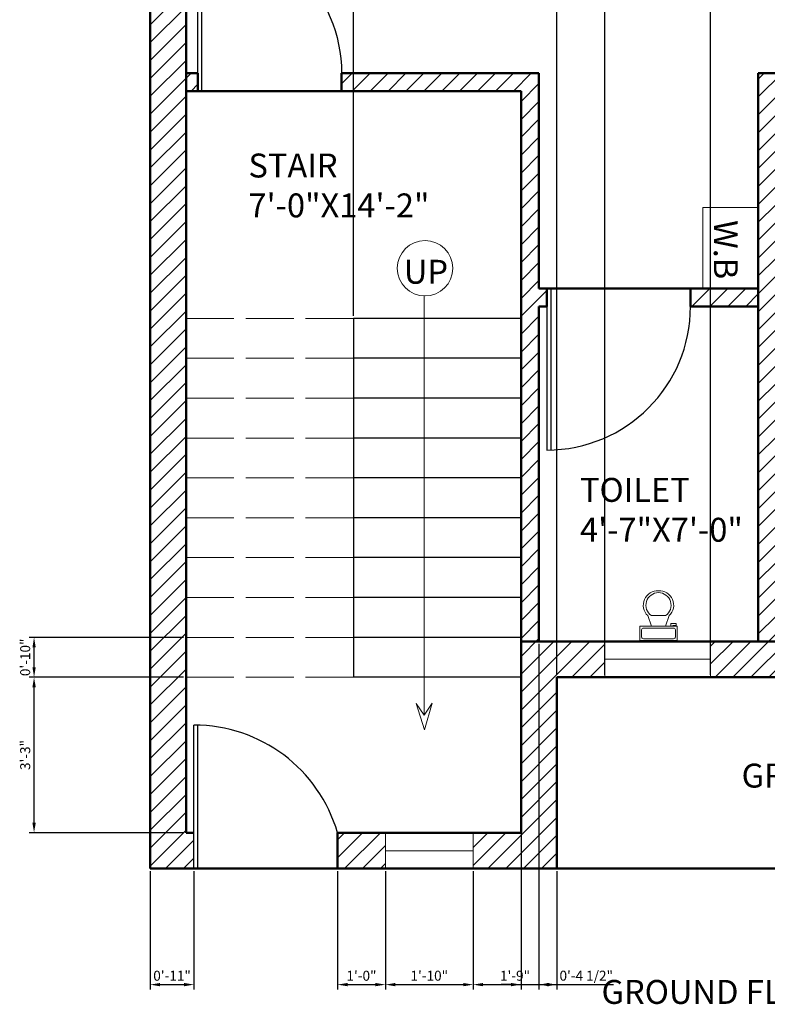
# Model space of a CAD drawing. Units: inches. Extents: x 3887 to 4286, y 884 to 1458.
# Tile 1 of 4: x 3889 to 4077, y 884 to 1131. Entities that reach past the tile are written whole.
import ezdxf

# ---------------------------------------------------------------- set-up
doc = ezdxf.new("R2010")
doc.units = ezdxf.units.IN
doc.linetypes.add('ACAD_ISO02W100', pattern=[15, 12, -3])
for name, color, linetype, lineweight in [('A-ANNO-DIMS', 2, 'Continuous', 18), ('A-ANNO-SYMB', 7, 'Continuous', 18), ('A-ANNO-TEXT', 7, 'Continuous', 25), ('A-AREA-IDEN', 7, 'Continuous', 25), ('A-DOOR', 3, 'Continuous', 25), ('A-FLOR-FIXT', 8, 'Continuous', 18), ('A-FLOR-STRS', 7, 'Continuous', 25), ('A-FLOR-STRS-OVHD', 8, 'ACAD_ISO02W100', 18), ('A-GLAZ', 4, 'Continuous', 18), ('A-WALL', 7, 'Continuous', 50), ('A-WALL-PATT', 252, 'Continuous', 13)]:
    doc.layers.add(name, color=color, linetype=linetype, lineweight=lineweight)
doc.styles.get("Standard").update_dxf_attribs({"font": 'arial.ttf'})
doc.dimstyles.new('ISO-25', dxfattribs={"dimtxt": 2.5, "dimasz": 2.5, "dimexe": 1.25, "dimexo": 0.625, "dimtad": 1, "dimdec": 0, "dimlunit": 3, "dimtxsty": 'Standard', "dimcen": 2.5, "dimadec": 0, "dimazin": 0, "dimtfac": 1, "dimtdec": 0, "dimtmove": 0, "dimatfit": 3, "dimfxl": 1, "dimarcsym": 0})

# ---------------------------------------------------------------- blocks, each defined once
blk = doc.blocks.new('*U5')
for p, q in [((9.5, -6), (9.5, -2)), ((-10, -8.5), (-8, -8.5)), ((-10, -9.5), (-10, -8.5)), ((-7, -9.5), (-10, -9.5)), ((-8, -8.5), (-8, -8)), ((-7, -8), (-7, -9.5)), ((-4, -8), (-6, -14)), ((4, -8), (6, -14)), ((4, -14), (-4, -14))]:
    blk.add_line(p, q)
blk.add_lwpolyline([(10.5, -8), (10.5, 0), (-10.5, 0), (-10.5, -8)], close=True)
for points in [[(-9.5, -2), (-9.5, -6)], [(8.5, -1), (-8.5, -1)], [(-8.5, -7), (8.5, -7)]]:
    blk.add_lwpolyline(points)
for centre, radius, start, end in [((-8.625, -1.875), 0.8839, 81.8699, 188.1301), ((8.625, -1.875), 0.8839, 351.8699, 98.1301), ((-8.625, -6.125), 0.8839, 171.869898, 278.1301), ((8.625, -6.125), 0.8839, 261.8699, 8.1301), ((-0.4772, -19.9188), 8.0953, 133.01722, 273.38), ((0.0374, -19.8731), 7.127, 124.50543, 269.7), ((-0.0373, -19.8731), 7.127, 270.3, 55.4946), ((0.4773, -19.9188), 8.0953, 266.62, 46.9828)]:
    blk.add_arc(centre, radius, start, end)
blk = doc.blocks.new('DOOR-SWING-36IN')
for p, q in [((35, 0), (35, 40.5)), ((36, 4.5), (36, 40.5))]:
    blk.add_line(p, q)
blk.add_arc((36, 4.5), 36, 90, 180)
blk = doc.blocks.new('*D39')
at = {"layer": 'A-ANNO-DIMS', "color": 0, "lineweight": -2, "transparency": 16777216}
for p, q in [((4015.18, 974.02), (4015.18, 887.29)), ((4019.68, 974.02), (4019.68, 887.29)), ((4012.68, 888.54), (4010.18, 888.54)), ((4015.18, 888.54), (4019.68, 888.54)), ((4022.18, 888.54), (4038.41, 888.54))]:
    blk.add_line(p, q, dxfattribs=at)
at = {"layer": 'A-ANNO-DIMS', "color": 0, "transparency": 16777216}
for points in [[(4012.68, 888.96), (4012.68, 888.13), (4015.18, 888.54)], [(4022.18, 888.96), (4022.18, 888.13), (4019.68, 888.54)]]:
    blk.add_solid(points, dxfattribs=at)
at = {"layer": 'Defpoints', "color": 0, "transparency": 16777216}
for p in [(4015.18, 974.64), (4019.68, 974.64), (4019.68, 888.54)]:
    blk.add_point(p, dxfattribs=at)
at = {"layer": 'A-ANNO-DIMS', "color": 0, "transparency": 16777216, "insert": (4031.54, 890.46), "char_height": 2.5, "attachment_point": 5}
blk.add_mtext('0\'-4 1/2"', dxfattribs=at)
blk = doc.blocks.new('*D40')
at = {"layer": 'A-ANNO-DIMS', "color": 0, "lineweight": -2, "transparency": 16777216}
for p, q in [((3922.18, 917.02), (3922.18, 887.29)), ((3933.18, 917.02), (3933.18, 887.29)), ((3924.68, 888.54), (3930.68, 888.54))]:
    blk.add_line(p, q, dxfattribs=at)
at = {"layer": 'A-ANNO-DIMS', "color": 0, "transparency": 16777216}
for points in [[(3924.68, 888.96), (3924.68, 888.13), (3922.18, 888.54)], [(3930.68, 888.96), (3930.68, 888.13), (3933.18, 888.54)]]:
    blk.add_solid(points, dxfattribs=at)
at = {"layer": 'Defpoints', "color": 0, "transparency": 16777216}
for p in [(3922.18, 917.64), (3933.18, 917.64), (3933.18, 888.54)]:
    blk.add_point(p, dxfattribs=at)
at = {"layer": 'A-ANNO-DIMS', "color": 0, "transparency": 16777216, "insert": (3927.68, 890.45), "char_height": 2.5, "attachment_point": 5}
blk.add_mtext('0\'-11"', dxfattribs=at)
blk = doc.blocks.new('*D41')
at = {"layer": 'A-ANNO-DIMS', "color": 0, "lineweight": -2, "transparency": 16777216}
for p, q in [((3969.18, 917.02), (3969.18, 887.29)), ((3981.18, 917.02), (3981.18, 887.29)), ((3971.68, 888.54), (3978.68, 888.54))]:
    blk.add_line(p, q, dxfattribs=at)
at = {"layer": 'A-ANNO-DIMS', "color": 0, "transparency": 16777216}
for points in [[(3971.68, 888.96), (3971.68, 888.13), (3969.18, 888.54)], [(3978.68, 888.96), (3978.68, 888.13), (3981.18, 888.54)]]:
    blk.add_solid(points, dxfattribs=at)
at = {"layer": 'Defpoints', "color": 0, "transparency": 16777216}
for p in [(3969.18, 917.64), (3981.18, 917.64), (3981.18, 888.54)]:
    blk.add_point(p, dxfattribs=at)
at = {"layer": 'A-ANNO-DIMS', "color": 0, "transparency": 16777216, "insert": (3975.18, 890.45), "char_height": 2.5, "attachment_point": 5}
blk.add_mtext('1\'-0"', dxfattribs=at)
blk = doc.blocks.new('*D43')
at = {"layer": 'A-ANNO-DIMS', "color": 0, "lineweight": -2, "transparency": 16777216}
for p, q in [((3981.18, 917.02), (3981.18, 887.29)), ((4003.18, 917.02), (4003.18, 887.29)), ((3983.68, 888.54), (4000.68, 888.54))]:
    blk.add_line(p, q, dxfattribs=at)
at = {"layer": 'A-ANNO-DIMS', "color": 0, "transparency": 16777216}
for points in [[(3983.68, 888.96), (3983.68, 888.13), (3981.18, 888.54)], [(4000.68, 888.96), (4000.68, 888.13), (4003.18, 888.54)]]:
    blk.add_solid(points, dxfattribs=at)
at = {"layer": 'Defpoints', "color": 0, "transparency": 16777216}
for p in [(3981.18, 917.64), (4003.18, 917.64), (4003.18, 888.54)]:
    blk.add_point(p, dxfattribs=at)
at = {"layer": 'A-ANNO-DIMS', "color": 0, "transparency": 16777216, "insert": (3992.18, 890.45), "char_height": 2.5, "attachment_point": 5}
blk.add_mtext('1\'-10"', dxfattribs=at)
blk = doc.blocks.new('*D44')
at = {"layer": 'A-ANNO-DIMS', "color": 0, "lineweight": -2, "transparency": 16777216}
for p, q in [((4003.18, 917.02), (4003.18, 887.29)), ((4024.18, 917.02), (4024.18, 887.29)), ((4005.68, 888.54), (4021.68, 888.54))]:
    blk.add_line(p, q, dxfattribs=at)
at = {"layer": 'A-ANNO-DIMS', "color": 0, "transparency": 16777216}
for points in [[(4005.68, 888.96), (4005.68, 888.13), (4003.18, 888.54)], [(4021.68, 888.96), (4021.68, 888.13), (4024.18, 888.54)]]:
    blk.add_solid(points, dxfattribs=at)
at = {"layer": 'Defpoints', "color": 0, "transparency": 16777216}
for p in [(4003.18, 917.64), (4024.18, 917.64), (4024.18, 888.54)]:
    blk.add_point(p, dxfattribs=at)
at = {"layer": 'A-ANNO-DIMS', "color": 0, "transparency": 16777216, "insert": (4013.68, 890.45), "char_height": 2.5, "attachment_point": 5}
blk.add_mtext('1\'-9"', dxfattribs=at)
blk = doc.blocks.new('*D45')
at = {"layer": 'A-ANNO-DIMS', "color": 0, "lineweight": -2, "transparency": 16777216}
for p, q in [((4024.18, 966.27), (4024.18, 1424.99)), ((4026.68, 1423.74), (4033.68, 1423.74)), ((4036.18, 966.27), (4036.18, 1424.99))]:
    blk.add_line(p, q, dxfattribs=at)
at = {"layer": 'A-ANNO-DIMS', "color": 0, "transparency": 16777216}
for points in [[(4026.68, 1424.16), (4026.68, 1423.33), (4024.18, 1423.74)], [(4033.68, 1424.16), (4033.68, 1423.33), (4036.18, 1423.74)]]:
    blk.add_solid(points, dxfattribs=at)
at = {"layer": 'Defpoints', "color": 0, "transparency": 16777216}
for p in [(4036.18, 1423.74), (4024.18, 965.64), (4036.18, 965.64)]:
    blk.add_point(p, dxfattribs=at)
at = {"layer": 'A-ANNO-DIMS', "color": 0, "transparency": 16777216, "insert": (4030.18, 1425.65), "char_height": 2.5, "attachment_point": 5}
blk.add_mtext('1\'-0"', dxfattribs=at)
blk = doc.blocks.new('*D46')
at = {"layer": 'A-ANNO-DIMS', "color": 0, "lineweight": -2, "transparency": 16777216}
for p, q in [((4036.18, 966.27), (4036.18, 1424.99)), ((4038.68, 1423.74), (4060.18, 1423.74)), ((4062.68, 966.27), (4062.68, 1424.99))]:
    blk.add_line(p, q, dxfattribs=at)
at = {"layer": 'A-ANNO-DIMS', "color": 0, "transparency": 16777216}
for points in [[(4038.68, 1424.16), (4038.68, 1423.33), (4036.18, 1423.74)], [(4060.18, 1424.16), (4060.18, 1423.33), (4062.68, 1423.74)]]:
    blk.add_solid(points, dxfattribs=at)
at = {"layer": 'Defpoints', "color": 0, "transparency": 16777216}
for p in [(4062.68, 1423.74), (4036.18, 965.64), (4062.68, 965.64)]:
    blk.add_point(p, dxfattribs=at)
at = {"layer": 'A-ANNO-DIMS', "color": 0, "transparency": 16777216, "insert": (4049.43, 1425.66), "char_height": 2.5, "attachment_point": 5}
blk.add_mtext('2\'-2 1/2"', dxfattribs=at)
blk = doc.blocks.new('*D47')
at = {"layer": 'A-ANNO-DIMS', "color": 0, "lineweight": -2, "transparency": 16777216}
for p, q in [((3930.56, 975.64), (3891.83, 975.64)), ((3893.08, 968.14), (3893.08, 973.14)), ((3930.56, 965.64), (3891.83, 965.64))]:
    blk.add_line(p, q, dxfattribs=at)
at = {"layer": 'A-ANNO-DIMS', "color": 0, "transparency": 16777216}
for points in [[(3892.67, 973.14), (3893.5, 973.14), (3893.08, 975.64)], [(3892.67, 968.14), (3893.5, 968.14), (3893.08, 965.64)]]:
    blk.add_solid(points, dxfattribs=at)
at = {"layer": 'Defpoints', "color": 0, "transparency": 16777216}
for p in [(3893.08, 975.64), (3931.18, 975.64), (3931.18, 965.64)]:
    blk.add_point(p, dxfattribs=at)
at = {"layer": 'A-ANNO-DIMS', "color": 0, "transparency": 16777216, "insert": (3891.18, 970.64), "char_height": 2.5, "attachment_point": 5, "rotation": 90}
blk.add_mtext('0\'-10"', dxfattribs=at)
blk = doc.blocks.new('*D52')
at = {"layer": 'A-ANNO-DIMS', "color": 0, "lineweight": -2, "transparency": 16777216}
for p, q in [((3931.18, 1056.27), (3931.18, 1424.99)), ((3933.68, 1423.74), (3970.68, 1423.74)), ((3973.18, 1056.27), (3973.18, 1424.99))]:
    blk.add_line(p, q, dxfattribs=at)
at = {"layer": 'A-ANNO-DIMS', "color": 0, "transparency": 16777216}
for points in [[(3933.68, 1424.16), (3933.68, 1423.33), (3931.18, 1423.74)], [(3970.68, 1424.16), (3970.68, 1423.33), (3973.18, 1423.74)]]:
    blk.add_solid(points, dxfattribs=at)
at = {"layer": 'Defpoints', "color": 0, "transparency": 16777216}
for p in [(3973.18, 1423.74), (3931.18, 1055.64), (3973.18, 1055.64)]:
    blk.add_point(p, dxfattribs=at)
at = {"layer": 'A-ANNO-DIMS', "color": 0, "transparency": 16777216, "insert": (3952.18, 1425.65), "char_height": 2.5, "attachment_point": 5}
blk.add_mtext('3\'-6"', dxfattribs=at)
blk = doc.blocks.new('*D53')
at = {"layer": 'A-ANNO-DIMS', "color": 0, "lineweight": -2, "transparency": 16777216}
for p, q in [((3930.56, 965.64), (3891.83, 965.64)), ((3893.08, 929.14), (3893.08, 963.14)), ((3930.56, 926.64), (3891.83, 926.64))]:
    blk.add_line(p, q, dxfattribs=at)
at = {"layer": 'A-ANNO-DIMS', "color": 0, "transparency": 16777216}
for points in [[(3892.67, 963.14), (3893.5, 963.14), (3893.08, 965.64)], [(3892.67, 929.14), (3893.5, 929.14), (3893.08, 926.64)]]:
    blk.add_solid(points, dxfattribs=at)
at = {"layer": 'Defpoints', "color": 0, "transparency": 16777216}
for p in [(3893.08, 965.64), (3931.18, 965.64), (3931.18, 926.64)]:
    blk.add_point(p, dxfattribs=at)
at = {"layer": 'A-ANNO-DIMS', "color": 0, "transparency": 16777216, "insert": (3891.18, 946.14), "char_height": 2.5, "attachment_point": 5, "rotation": 90}
blk.add_mtext('3\'-3"', dxfattribs=at)

msp = doc.modelspace()

# ---------------------------------------------------------------- hatches: boundary and pattern name
at = {"layer": 'A-WALL-PATT'}
h = msp.add_hatch(dxfattribs=at)
h.set_pattern_fill('ANSI31', color=256)
h.paths.add_polyline_path([(4079.68, 1394.64), (3922.18, 1394.64), (3922.18, 1343.64), (3931.18, 1343.64), (3931.18, 1385.64), (4079.68, 1385.64)])
h.paths.add_polyline_path([(4156.18, 1394.64), (4109.68, 1394.64), (4109.68, 1385.64), (4156.18, 1385.64)])
h.paths.add_polyline_path([(4255.18, 1394.64), (4216.18, 1394.64), (4216.18, 1385.64), (4246.18, 1385.64), (4246.18, 1343.64), (4255.18, 1343.64)])
h.paths.add_polyline_path([(3931.18, 1283.64), (3922.18, 1283.64), (3922.18, 1207.14), (3931.18, 1207.14)])
h.paths.add_polyline_path([(4024.18, 1241.64), (3931.18, 1241.64), (3931.18, 1237.14), (4024.18, 1237.14)])
h.paths.add_polyline_path([(4067.68, 1291.14), (4079.68, 1291.14), (4079.68, 1295.64), (4067.68, 1295.64), (4067.68, 1385.64), (4063.18, 1385.64), (4063.18, 1241.64), (4060.18, 1241.64), (4060.18, 1237.14), (4067.68, 1237.14)])
h.paths.add_polyline_path([(4126.18, 1385.64), (4121.68, 1385.64), (4121.68, 1295.64), (4109.68, 1295.64), (4109.68, 1291.14), (4121.68, 1291.14), (4121.68, 1280.64), (4126.18, 1280.64)])
h.paths.add_polyline_path([(4246.18, 1241.64), (4126.18, 1241.64), (4126.18, 1244.64), (4121.68, 1244.64), (4121.68, 1156.14), (4126.18, 1156.14), (4126.18, 1237.14), (4246.18, 1237.14)])
h.paths.add_polyline_path([(4255.18, 1283.64), (4246.18, 1283.64), (4246.18, 1210.14), (4255.18, 1210.14)])
h.paths.add_polyline_path([(4255.18, 1150.14), (4246.18, 1150.14), (4246.18, 1073.64), (4255.18, 1073.64)])
h.paths.add_polyline_path([(4246.18, 1117.14), (4126.18, 1117.14), (4126.18, 1120.14), (4121.68, 1120.14), (4121.68, 1117.14), (4119.68, 1117.14), (4119.68, 1112.64), (4246.18, 1112.64)])
h.paths.add_polyline_path([(4079.18, 1112.64), (4083.68, 1112.64), (4083.68, 1117.14), (4074.68, 1117.14), (4074.68, 974.64), (4079.18, 974.64)])
h.paths.add_polyline_path([(4019.68, 1117.14), (3970.18, 1117.14), (3970.18, 1112.64), (4015.18, 1112.64), (4015.18, 974.64), (4019.68, 974.64), (4019.68, 1058.64), (4021.68, 1058.64), (4021.68, 1063.14), (4019.68, 1063.14)])
h.paths.add_polyline_path([(3931.18, 1147.14), (3922.18, 1147.14), (3922.18, 917.64), (3933.18, 917.64), (3933.18, 926.64), (3931.18, 926.64)])
h.paths.add_polyline_path([(4024.18, 965.64), (4036.18, 965.64), (4036.18, 974.64), (4015.18, 974.64), (4015.18, 926.64), (4003.18, 926.64), (4003.18, 917.64), (4024.18, 917.64)])
h.paths.add_polyline_path([(4132.68, 974.64), (4062.68, 974.64), (4062.68, 965.64), (4132.68, 965.64)])
h.paths.add_polyline_path([(4255.18, 1013.64), (4246.18, 1013.64), (4246.18, 974.64), (4192.68, 974.64), (4192.68, 965.64), (4255.18, 965.64)])
h = msp.add_hatch(dxfattribs=at)
h.set_pattern_fill('ANSI31', color=256)
h.paths.add_polyline_path([(3934.18, 1117.14), (3931.18, 1117.14), (3931.18, 1112.64), (3934.18, 1112.64)])
h.paths.add_polyline_path([(3981.18, 926.64), (3969.18, 926.64), (3969.18, 917.64), (3981.18, 917.64)])
h = msp.add_hatch(dxfattribs=at)
h.set_pattern_fill('ANSI31', color=256)
h.paths.add_polyline_path([(4074.68, 1063.14), (4057.68, 1063.14), (4057.68, 1058.64), (4074.68, 1058.64)])

# ---------------------------------------------------------------- linework, layer by layer
at = {"layer": 'A-ANNO-SYMB'}
for p, q in [((3990.92, 1061.3), (3990.92, 956.09)), ((3990.92, 956.09), (3988.9, 959.07)), ((3988.9, 959.07), (3990.95, 952.49)), ((3990.92, 956.09), (3992.89, 959.11)), ((3992.89, 959.11), (3990.95, 952.49))]:
    msp.add_line(p, q, dxfattribs=at)
msp.add_circle((3991.11, 1068.24), 6.95, dxfattribs=at)
at = {"layer": 'A-DOOR'}
for p, q in [((3933.18, 917.64), (3933.18, 953.64)), ((3934.18, 917.64), (3934.18, 953.64))]:
    msp.add_line(p, q, dxfattribs=at)
msp.add_arc((3933.18, 916.14), 37.5, 16.2602, 90, dxfattribs=at)
at = {"layer": 'A-FLOR-FIXT'}
for p, q in [((4060.74, 1063.14), (4060.74, 1083.46)), ((4060.74, 1083.46), (4074.68, 1083.46))]:
    msp.add_line(p, q, dxfattribs=at)
at = {"layer": 'A-FLOR-STRS'}
for p, q in [((3973.18, 1055.64), (3973.18, 965.64)), ((4015.18, 1055.64), (3973.18, 1055.64)), ((4015.18, 1045.64), (3973.18, 1045.64)), ((4015.18, 1035.64), (3973.18, 1035.64)), ((4015.18, 1025.64), (3973.18, 1025.64)), ((4015.18, 1015.64), (3973.18, 1015.64)), ((4015.18, 1005.64), (3973.18, 1005.64)), ((4015.18, 1005.64), (3973.18, 1005.64)), ((4015.18, 995.64), (3973.18, 995.64)), ((4015.18, 985.64), (3973.18, 985.64)), ((4015.18, 975.64), (3973.18, 975.64)), ((4015.18, 965.64), (3973.18, 965.64))]:
    msp.add_line(p, q, dxfattribs=at)
at = {"layer": 'A-FLOR-STRS-OVHD'}
for p, q in [((3973.18, 1055.64), (3931.18, 1055.64)), ((3973.18, 1045.64), (3931.18, 1045.64)), ((3973.18, 1035.64), (3931.18, 1035.64)), ((3973.18, 1025.64), (3931.18, 1025.64)), ((3973.18, 1015.64), (3931.18, 1015.64)), ((3973.18, 1005.64), (3931.18, 1005.64)), ((3973.18, 995.64), (3931.18, 995.64)), ((3973.18, 985.64), (3931.18, 985.64)), ((3973.18, 975.64), (3931.18, 975.64)), ((3973.18, 965.64), (3931.18, 965.64))]:
    msp.add_line(p, q, dxfattribs=at)
at = {"layer": 'A-GLAZ'}
for p, q in [((4036.18, 965.64), (4036.18, 974.64)), ((4062.68, 974.64), (4062.68, 965.64)), ((4036.18, 970.14), (4062.68, 970.14)), ((3981.18, 926.64), (3981.18, 917.64)), ((4003.18, 926.64), (4003.18, 917.64)), ((3981.18, 922.14), (4003.18, 922.14))]:
    msp.add_line(p, q, dxfattribs=at)
at = {"layer": 'A-WALL'}
for p, q in [((3922.18, 1394.64), (3922.18, 917.64)), ((3931.18, 1385.64), (3931.18, 926.64)), ((3931.18, 1117.14), (3934.18, 1117.14)), ((3934.18, 1117.14), (3934.18, 1112.64)), ((3970.18, 1112.64), (3970.18, 1117.14)), ((3970.18, 1117.14), (4019.68, 1117.14)), ((4019.68, 1117.14), (4019.68, 1063.14)), ((4074.68, 1117.14), (4074.68, 974.64)), ((4074.68, 1117.14), (4121.68, 1117.14)), ((3931.18, 1112.64), (4015.18, 1112.64)), ((4015.18, 1112.64), (4015.18, 926.64)), ((4019.68, 1063.14), (4074.68, 1063.14)), ((4021.68, 1058.64), (4021.68, 1063.14)), ((4057.68, 1063.14), (4057.68, 1058.64)), ((4019.68, 1058.64), (4021.68, 1058.64)), ((4019.68, 1058.64), (4019.68, 974.64)), ((4057.68, 1058.64), (4074.68, 1058.64)), ((4015.18, 974.64), (4246.18, 974.64)), ((4024.18, 965.64), (4255.18, 965.64)), ((4024.18, 965.64), (4024.18, 917.64)), ((3931.18, 926.64), (3933.18, 926.64)), ((3969.18, 917.64), (3969.18, 926.64)), ((3969.18, 926.64), (4015.18, 926.64)), ((3922.18, 917.64), (4255.18, 917.64))]:
    msp.add_line(p, q, dxfattribs=at)

# ---------------------------------------------------------------- block references
at = {"layer": 'A-DOOR', "extrusion": (0, 0, -1), "zscale": -1}
msp.add_blockref('DOOR-SWING-36IN', (-3970.18, 1112.64), dxfattribs=at)
at = {"layer": 'A-DOOR', "rotation": 180}
msp.add_blockref('DOOR-SWING-36IN', (4057.68, 1063.14), dxfattribs=at)
at = {"layer": 'A-FLOR-FIXT', "xscale": 0.4449568002020858, "yscale": 0.4449568002020858, "zscale": 0.4449568002020858, "rotation": 180}
msp.add_blockref('*U5', (4049.65, 974.86), dxfattribs=at)

# ---------------------------------------------------------------- texts
at = {"layer": 'A-ANNO-TEXT', "insert": (4069.53, 1080.31), "char_height": 6, "attachment_point": 1, "rotation": 270}
msp.add_mtext_dynamic_manual_height_columns('W.B', width=8.3813, gutter_width=12.5, heights=[0], dxfattribs=at)
at = {"layer": 'A-ANNO-TEXT', "insert": (3985.8, 1070.35), "char_height": 6, "attachment_point": 1}
msp.add_mtext_dynamic_manual_height_columns('UP', width=9.7205, gutter_width=12.5, heights=[0], dxfattribs=at)
at = {"layer": 'A-ANNO-TEXT', "insert": (4035.36, 889.71), "char_height": 6, "width": 97.9816, "attachment_point": 1}
msp.add_mtext('GROUND FLOOR PLAN', dxfattribs=at)
at = {"layer": 'A-AREA-IDEN', "char_height": 6, "attachment_point": 1}
for s, width, insert in [('STAIR\\P7\'-0"X14\'-2"', 7.3337, (3946.83, 1097)), ('TOILET\\P4\'-7"X7\'-0"', 6, (4029.96, 1015.64))]:
    msp.add_mtext_dynamic_manual_height_columns(s, width=width, gutter_width=12.5, heights=[0], dxfattribs=dict(at, insert=insert))
at = {"layer": 'A-AREA-IDEN', "insert": (4070.48, 943.97), "char_height": 6, "attachment_point": 1}
msp.add_mtext('GREENARY', dxfattribs=at)

# ---------------------------------------------------------------- dimensions: what is measured, and where the dimension line sits
at = {"layer": 'A-ANNO-DIMS'}
for base, p1, p2, picture, middle in [((4062.68, 1423.74), (4036.18, 965.64), (4062.68, 965.64), '*D46', (4049.43, 1425.66)), ((3973.18, 1423.74), (3931.18, 1055.64), (3973.18, 1055.64), '*D52', (3952.18, 1425.65)), ((4036.18, 1423.74), (4024.18, 965.64), (4036.18, 965.64), '*D45', (4030.18, 1425.65)), ((4019.68, 888.54), (4015.18, 974.64), (4019.68, 974.64), '*D39', (4031.54, 890.46)), ((3933.18, 888.54), (3922.18, 917.64), (3933.18, 917.64), '*D40', (3927.68, 890.45)), ((3981.18, 888.54), (3969.18, 917.64), (3981.18, 917.64), '*D41', (3975.18, 890.45)), ((4003.18, 888.54), (3981.18, 917.64), (4003.18, 917.64), '*D43', (3992.18, 890.45)), ((4024.18, 888.54), (4003.18, 917.64), (4024.18, 917.64), '*D44', (4013.68, 890.45))]:
    dim = msp.add_linear_dim(base=base, p1=p1, p2=p2, dimstyle='ISO-25', override={"dimdec": 1, "dimlfac": 1, "dimrnd": 0, "dimzin": 1, "dimdsep": 46, "dimlunit": 4, "dimfrac": 2}, dxfattribs=at)
    dim.commit()
    dim.dimension.update_dxf_attribs({"geometry": picture, "text_midpoint": middle})
for base, p1, p2, picture, middle in [((3893.08, 975.64), (3931.18, 965.64), (3931.18, 975.64), '*D47', (3891.18, 970.64)), ((3893.08, 965.64), (3931.18, 926.64), (3931.18, 965.64), '*D53', (3891.18, 946.14))]:
    dim = msp.add_linear_dim(base=base, p1=p1, p2=p2, angle=90, dimstyle='ISO-25', override={"dimdec": 1, "dimlfac": 1, "dimrnd": 0, "dimzin": 1, "dimdsep": 46, "dimlunit": 4, "dimfrac": 2}, dxfattribs=at)
    dim.commit()
    dim.dimension.update_dxf_attribs({"geometry": picture, "text_midpoint": middle})

doc.saveas('drawing.dxf')
